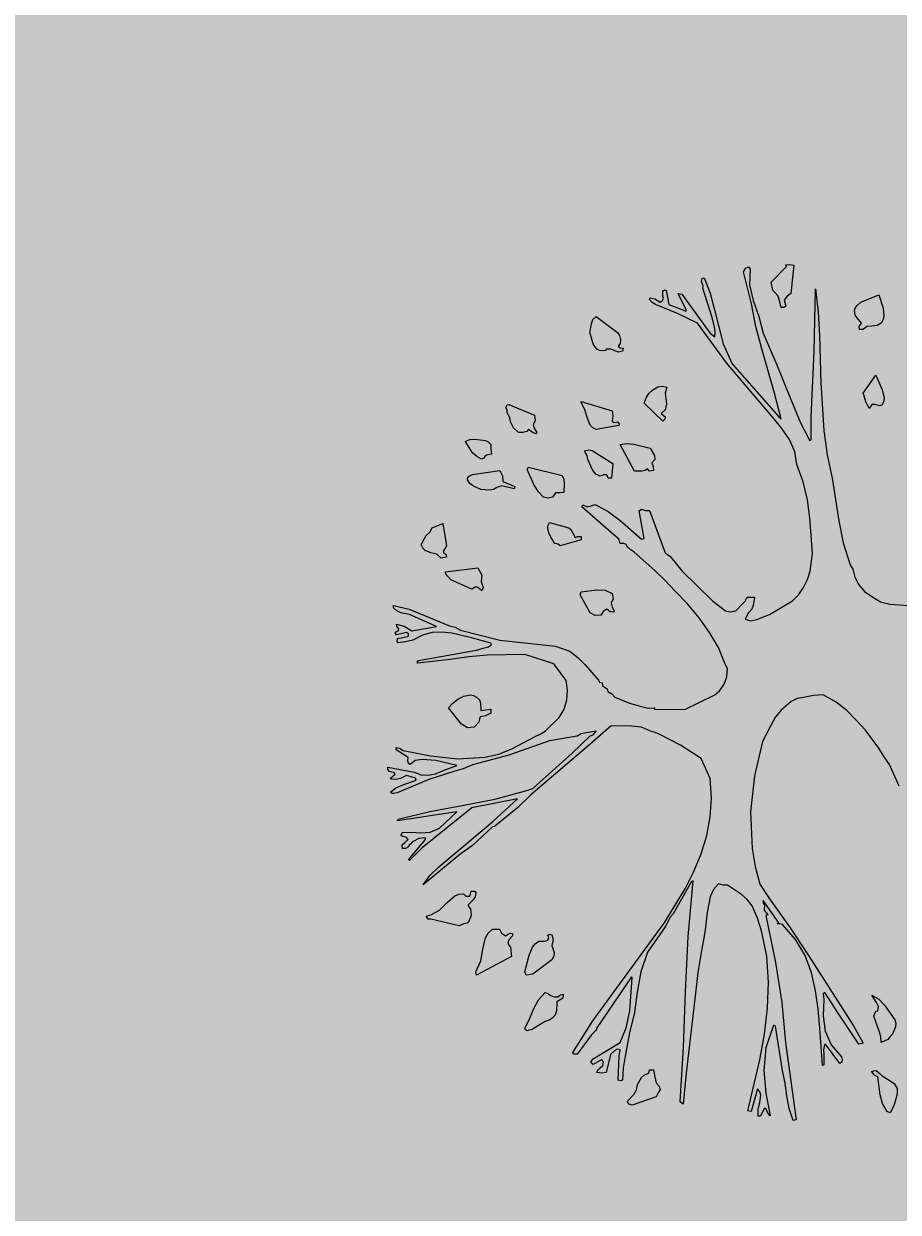
# Model space of a CAD drawing. Units: inches. Extents: x 84 to 1044, y -280 to 906.
# Tile 99 of 105: x 861 to 885, y 445 to 478. Entities that reach past the tile are written whole.
import ezdxf

# ---------------------------------------------------------------- set-up
doc = ezdxf.new("R2010")
doc.units = ezdxf.units.IN
doc.layers.add('A-ANNO-DIMS', color=2, linetype='Continuous', lineweight=18)
doc.layers.add('L-PLNT', color=114, linetype='Continuous', lineweight=15)
doc.layers.add('L-PLNT-PATT', color=9, linetype='Continuous', lineweight=9, true_color=0xafd9aa)
doc.styles.get("Standard").update_dxf_attribs({"font": 'arial.ttf'})
doc.dimstyles.get("Standard").update_dxf_attribs({"dimtxt": 0.18, "dimasz": 0.18, "dimexe": 0.18, "dimexo": 0.0625, "dimgap": 0.09, "dimtad": 0, "dimtih": 1, "dimtoh": 1, "dimdec": 4, "dimzin": 0, "dimdsep": 46, "dimtxsty": 'Standard', "dimcen": 0.09, "dimadec": 0, "dimazin": 0, "dimtfac": 1, "dimtdec": 4, "dimtofl": 0, "dimtmove": 0, "dimatfit": 3, "dimfxl": 1, "dimtolj": 1, "dimtzin": 0, "dimarcsym": 0})

# ---------------------------------------------------------------- blocks, each defined once
blk = doc.blocks.new('A$C37E508DF')
for p, q in [((0.7083, 1.5239), (0.7152, 1.5244)), ((0.7096, 1.5209), (0.7083, 1.5239)), ((0.7152, 1.5244), (0.7225, 1.5231)), ((0.6329, 1.5111), (0.6367, 1.5175)), ((0.6475, 1.4545), (0.6329, 1.5111)), ((0.6367, 1.5175), (0.6423, 1.5201)), ((0.6423, 1.5201), (0.6453, 1.5158)), ((0.6453, 1.5158), (0.644, 1.4879)), ((0.6826, 1.493), (0.7096, 1.5209)), ((0.7225, 1.5231), (0.7174, 1.4729)), ((0.5583, 1.4948), (0.5596, 1.4995)), ((0.5596, 1.4905), (0.5583, 1.4948)), ((0.5596, 1.4995), (0.563, 1.5003)), ((0.5613, 1.4862), (0.5596, 1.4905)), ((0.5608, 1.4823), (0.5613, 1.4862)), ((0.5767, 1.4317), (0.5608, 1.4823)), ((0.563, 1.5003), (0.5737, 1.4733)), ((0.644, 1.4879), (0.6505, 1.46)), ((0.6852, 1.4785), (0.6826, 1.493)), ((0.4657, 1.4622), (0.4669, 1.4652)), ((0.4708, 1.4566), (0.4657, 1.4622)), ((0.4669, 1.4652), (0.4755, 1.463)), ((0.4755, 1.463), (0.4845, 1.4575)), ((0.4884, 1.4596), (0.4905, 1.4635)), ((0.4897, 1.4772), (0.4935, 1.4789)), ((0.4897, 1.4678), (0.4897, 1.4772)), ((0.4905, 1.4635), (0.4897, 1.4678)), ((0.4935, 1.4789), (0.4952, 1.478)), ((0.4952, 1.478), (0.5004, 1.4532)), ((0.5313, 1.4437), (0.5167, 1.4729)), ((0.5167, 1.4729), (0.5231, 1.4716)), ((0.5231, 1.4716), (0.5686, 1.409)), ((0.5737, 1.4733), (0.5814, 1.4437)), ((0.6946, 1.4682), (0.6852, 1.4785)), ((0.6976, 1.4579), (0.6946, 1.4682)), ((0.7109, 1.4682), (0.7053, 1.4609)), ((0.7053, 1.4609), (0.7083, 1.4502)), ((0.7174, 1.4729), (0.7109, 1.4682)), ((0.7589, 1.3691), (0.7615, 1.481)), ((0.7615, 1.481), (0.7658, 1.4395)), ((0.8421, 1.4575), (0.8739, 1.4703)), ((0.8739, 1.4703), (0.882, 1.4463)), ((0.4764, 1.4532), (0.4708, 1.4566)), ((0.5154, 1.4373), (0.4764, 1.4532)), ((0.4845, 1.4575), (0.4884, 1.4596)), ((0.5004, 1.4532), (0.5308, 1.4412)), ((0.5308, 1.4412), (0.5313, 1.4437)), ((0.5814, 1.4437), (0.5969, 1.3833)), ((0.6552, 1.4137), (0.6475, 1.4545)), ((0.6505, 1.46), (0.6603, 1.4317)), ((0.7002, 1.4476), (0.6976, 1.4579)), ((0.7049, 1.448), (0.7002, 1.4476)), ((0.7083, 1.4502), (0.7049, 1.448)), ((0.7658, 1.4395), (0.7684, 1.3979)), ((0.831, 1.4424), (0.8323, 1.4476)), ((0.8318, 1.4343), (0.831, 1.4424)), ((0.8323, 1.4476), (0.8357, 1.451)), ((0.8357, 1.451), (0.8421, 1.4575)), ((0.882, 1.4463), (0.8829, 1.433)), ((0.3598, 1.403), (0.3628, 1.4189)), ((0.3628, 1.4189), (0.3649, 1.4266)), ((0.3649, 1.4266), (0.3709, 1.4317)), ((0.3709, 1.4317), (0.4086, 1.403)), ((0.551, 1.4197), (0.5154, 1.4373)), ((0.6029, 1.3494), (0.551, 1.4197)), ((0.5814, 1.4133), (0.5767, 1.4317)), ((0.6603, 1.4317), (0.668, 1.4021)), ((0.8353, 1.4292), (0.8318, 1.4343)), ((0.8434, 1.4197), (0.8353, 1.4292)), ((0.8391, 1.4141), (0.8434, 1.4197)), ((0.8781, 1.4197), (0.8709, 1.4154)), ((0.8816, 1.4262), (0.8781, 1.4197)), ((0.8829, 1.433), (0.8816, 1.4262)), ((0.3602, 1.4021), (0.3598, 1.403)), ((0.364, 1.3888), (0.3602, 1.4021)), ((0.4086, 1.403), (0.4125, 1.3979)), ((0.4125, 1.3979), (0.4142, 1.391)), ((0.5686, 1.409), (0.5741, 1.4021)), ((0.5741, 1.4021), (0.5823, 1.3953)), ((0.5827, 1.4043), (0.5814, 1.4133)), ((0.5823, 1.3953), (0.5827, 1.4043)), ((0.6655, 1.3743), (0.6552, 1.4137)), ((0.668, 1.4021), (0.6925, 1.3455)), ((0.7684, 1.3979), (0.771, 1.3134)), ((0.8395, 1.4086), (0.8391, 1.4141)), ((0.846, 1.4086), (0.8395, 1.4086)), ((0.8528, 1.4137), (0.846, 1.4086)), ((0.8619, 1.4146), (0.8528, 1.4137)), ((0.8709, 1.4154), (0.8619, 1.4146)), ((0.3657, 1.3828), (0.364, 1.3888)), ((0.3683, 1.3781), (0.3657, 1.3828)), ((0.3718, 1.3738), (0.3683, 1.3781)), ((0.4134, 1.3837), (0.4099, 1.3781)), ((0.4099, 1.3781), (0.4134, 1.376)), ((0.4142, 1.391), (0.4134, 1.3837)), ((0.4134, 1.376), (0.4189, 1.3751)), ((0.5969, 1.3833), (0.6132, 1.3472)), ((0.3765, 1.3713), (0.3718, 1.3738)), ((0.3872, 1.3708), (0.3765, 1.3713)), ((0.3885, 1.3738), (0.3872, 1.3708)), ((0.3971, 1.3734), (0.3885, 1.3738)), ((0.4039, 1.3704), (0.3971, 1.3734)), ((0.4108, 1.3683), (0.4039, 1.3704)), ((0.4176, 1.37), (0.4108, 1.3683)), ((0.4189, 1.3751), (0.4176, 1.37)), ((0.6882, 1.2949), (0.6655, 1.3743)), ((0.7538, 1.2529), (0.7589, 1.3691)), ((0.6595, 1.2829), (0.6029, 1.3494)), ((0.6132, 1.3472), (0.6959, 1.2529)), ((0.6925, 1.3455), (0.7161, 1.2868)), ((0.771, 1.3134), (0.7761, 1.2285)), ((0.846, 1.2949), (0.8687, 1.3271)), ((0.8687, 1.3271), (0.8803, 1.3014)), ((0.4597, 1.2868), (0.4648, 1.2945)), ((0.4648, 1.2945), (0.4717, 1.3009)), ((0.4717, 1.3009), (0.4807, 1.3065)), ((0.4807, 1.3065), (0.4884, 1.3074)), ((0.4884, 1.3074), (0.4965, 1.3057)), ((0.4965, 1.3057), (0.4935, 1.2954)), ((0.4935, 1.2954), (0.4948, 1.2855)), ((0.7002, 1.2495), (0.6882, 1.2949)), ((0.8473, 1.2924), (0.846, 1.2949)), ((0.8507, 1.2795), (0.8473, 1.2924)), ((0.8803, 1.3014), (0.8833, 1.2872)), ((0.2101, 1.2696), (0.2127, 1.2744)), ((0.2127, 1.2744), (0.2152, 1.2752)), ((0.2152, 1.2752), (0.2611, 1.2559)), ((0.3439, 1.2804), (0.3992, 1.2636)), ((0.3439, 1.2787), (0.3439, 1.2804)), ((0.3507, 1.2662), (0.3439, 1.2787)), ((0.4562, 1.2774), (0.4597, 1.2868)), ((0.4897, 1.2452), (0.4562, 1.2774)), ((0.4961, 1.2756), (0.4935, 1.2658)), ((0.4948, 1.2855), (0.4961, 1.2756)), ((0.6865, 1.2508), (0.6595, 1.2829)), ((0.7161, 1.2868), (0.7349, 1.2422)), ((0.8567, 1.2679), (0.8507, 1.2795)), ((0.8619, 1.2752), (0.8567, 1.2679)), ((0.867, 1.2752), (0.8619, 1.2752)), ((0.8713, 1.2739), (0.867, 1.2752)), ((0.8756, 1.2726), (0.8713, 1.2739)), ((0.8799, 1.2744), (0.8756, 1.2726)), ((0.8829, 1.2808), (0.8799, 1.2744)), ((0.8833, 1.2872), (0.8829, 1.2808)), ((0.2127, 1.2654), (0.2101, 1.2696)), ((0.2127, 1.2602), (0.2127, 1.2654)), ((0.2174, 1.2521), (0.2127, 1.2602)), ((0.2182, 1.2443), (0.2174, 1.2521)), ((0.2611, 1.2559), (0.262, 1.2465)), ((0.3546, 1.2516), (0.3507, 1.2662)), ((0.3602, 1.2383), (0.3546, 1.2516)), ((0.3992, 1.2636), (0.4005, 1.2546)), ((0.4005, 1.2546), (0.3992, 1.2452)), ((0.4935, 1.2658), (0.4867, 1.2589)), ((0.4867, 1.2589), (0.4935, 1.2529)), ((0.4931, 1.2491), (0.4897, 1.2452)), ((0.4935, 1.2529), (0.4931, 1.2491)), ((0.7015, 1.2323), (0.6865, 1.2508)), ((0.6959, 1.2529), (0.7002, 1.2495)), ((0.7538, 1.2122), (0.7538, 1.2529)), ((0.2234, 1.2336), (0.2182, 1.2443)), ((0.2328, 1.2251), (0.2234, 1.2336)), ((0.2504, 1.2306), (0.2474, 1.2268)), ((0.2568, 1.2255), (0.2504, 1.2306)), ((0.262, 1.2465), (0.2586, 1.2388)), ((0.2586, 1.2388), (0.2611, 1.2319)), ((0.2611, 1.2319), (0.265, 1.2251)), ((0.3649, 1.2336), (0.3602, 1.2383)), ((0.3709, 1.2306), (0.3649, 1.2336)), ((0.4112, 1.2375), (0.3709, 1.2306)), ((0.3992, 1.2452), (0.4026, 1.2431)), ((0.4026, 1.2431), (0.4086, 1.2443)), ((0.4086, 1.2443), (0.4121, 1.2401)), ((0.4121, 1.2401), (0.4112, 1.2375)), ((0.7148, 1.2126), (0.7015, 1.2323)), ((0.7349, 1.2422), (0.7482, 1.216)), ((0.7761, 1.2285), (0.7821, 1.1856)), ((0.1376, 1.2092), (0.1458, 1.2126)), ((0.1389, 1.2079), (0.1376, 1.2092)), ((0.1505, 1.189), (0.1389, 1.2079)), ((0.1458, 1.2126), (0.1548, 1.2135)), ((0.1548, 1.2135), (0.1741, 1.2109)), ((0.1741, 1.2109), (0.1784, 1.2083)), ((0.1784, 1.2083), (0.1831, 1.204)), ((0.2401, 1.2251), (0.2328, 1.2251)), ((0.2474, 1.2268), (0.2401, 1.2251)), ((0.2633, 1.2229), (0.2568, 1.2255)), ((0.265, 1.2251), (0.2633, 1.2229)), ((0.7246, 1.1908), (0.7148, 1.2126)), ((0.7482, 1.216), (0.7508, 1.2109)), ((0.7508, 1.2109), (0.7538, 1.2122)), ((0.1582, 1.1822), (0.1505, 1.189)), ((0.1788, 1.1852), (0.1758, 1.1847)), ((0.1848, 1.1865), (0.1788, 1.1852)), ((0.1831, 1.204), (0.1831, 1.1959)), ((0.1831, 1.1959), (0.1848, 1.1865)), ((0.3507, 1.1916), (0.352, 1.1933)), ((0.355, 1.1839), (0.3507, 1.1916)), ((0.352, 1.1933), (0.3576, 1.1942)), ((0.3576, 1.1942), (0.364, 1.1929)), ((0.364, 1.1929), (0.4005, 1.1702)), ((0.4134, 1.204), (0.4258, 1.2058)), ((0.4391, 1.156), (0.4134, 1.204)), ((0.4258, 1.2058), (0.4382, 1.2045)), ((0.4382, 1.2045), (0.4669, 1.1972)), ((0.4669, 1.1972), (0.4747, 1.1843)), ((0.7281, 1.168), (0.7246, 1.1908)), ((0.7821, 1.1856), (0.7911, 1.1436)), ((0.1668, 1.1775), (0.1582, 1.1822)), ((0.1711, 1.1792), (0.1668, 1.1775)), ((0.1728, 1.1826), (0.1711, 1.1792)), ((0.1758, 1.1847), (0.1728, 1.1826)), ((0.3563, 1.177), (0.355, 1.1839)), ((0.3645, 1.1586), (0.3563, 1.177)), ((0.4005, 1.1702), (0.3979, 1.1436)), ((0.4751, 1.177), (0.47, 1.1714)), ((0.47, 1.1714), (0.4721, 1.1646)), ((0.4721, 1.1646), (0.473, 1.1573)), ((0.4747, 1.1843), (0.4751, 1.177)), ((0.7396, 1.1371), (0.7281, 1.168)), ((0.1419, 1.1436), (0.1449, 1.1474)), ((0.1419, 1.141), (0.1419, 1.1436)), ((0.1449, 1.1474), (0.1509, 1.1504)), ((0.1509, 1.1504), (0.1994, 1.1573)), ((0.1994, 1.1573), (0.2041, 1.1479)), ((0.2041, 1.1479), (0.2045, 1.138)), ((0.2478, 1.1594), (0.2504, 1.1637)), ((0.2607, 1.1316), (0.2478, 1.1594)), ((0.2504, 1.1637), (0.3104, 1.1487)), ((0.3104, 1.1487), (0.3134, 1.1423)), ((0.37, 1.1509), (0.3645, 1.1586)), ((0.3778, 1.1474), (0.37, 1.1509)), ((0.3842, 1.15), (0.3778, 1.1474)), ((0.3898, 1.15), (0.3842, 1.15)), ((0.3923, 1.1436), (0.3898, 1.15)), ((0.3979, 1.1436), (0.3923, 1.1436)), ((0.4519, 1.1564), (0.4391, 1.156)), ((0.458, 1.1573), (0.4519, 1.1564)), ((0.4622, 1.1607), (0.458, 1.1573)), ((0.4657, 1.156), (0.4622, 1.1607)), ((0.473, 1.1573), (0.4657, 1.156)), ((0.7911, 1.1436), (0.8027, 1.0677)), ((0.1462, 1.1342), (0.1419, 1.141)), ((0.1522, 1.1294), (0.1462, 1.1342)), ((0.1655, 1.1234), (0.1522, 1.1294)), ((0.181, 1.1226), (0.1655, 1.1234)), ((0.1878, 1.1234), (0.181, 1.1226)), ((0.1938, 1.1273), (0.1878, 1.1234)), ((0.2032, 1.1303), (0.1938, 1.1273)), ((0.2247, 1.1251), (0.2032, 1.1303)), ((0.2045, 1.138), (0.226, 1.129)), ((0.226, 1.129), (0.2247, 1.1251)), ((0.268, 1.1196), (0.2607, 1.1316)), ((0.3134, 1.1423), (0.3139, 1.1346)), ((0.3139, 1.1346), (0.3134, 1.1183)), ((0.7469, 1.1054), (0.7396, 1.1371)), ((0.277, 1.1101), (0.268, 1.1196)), ((0.2856, 1.108), (0.277, 1.1101)), ((0.2933, 1.1101), (0.2856, 1.108)), ((0.2959, 1.1144), (0.2933, 1.1101)), ((0.2984, 1.1179), (0.2959, 1.1144)), ((0.3066, 1.1179), (0.2984, 1.1179)), ((0.3134, 1.1183), (0.3066, 1.1179)), ((0.7512, 1.0728), (0.7469, 1.1054)), ((0.3456, 1.093), (0.3469, 1.0964)), ((0.3842, 1.0591), (0.3456, 1.093)), ((0.3469, 1.0964), (0.355, 1.093)), ((0.355, 1.093), (0.3619, 1.0943)), ((0.3619, 1.0943), (0.3692, 1.0968)), ((0.3692, 1.0968), (0.3923, 1.0844)), ((0.3923, 1.0844), (0.4129, 1.069)), ((0.4472, 1.0857), (0.4515, 1.0887)), ((0.4562, 1.0364), (0.4472, 1.0857)), ((0.4515, 1.0887), (0.4584, 1.0865)), ((0.4584, 1.0865), (0.4657, 1.0861)), ((0.4657, 1.0861), (0.4939, 1.0107)), ((0.0789, 1.0552), (0.0978, 1.063)), ((0.0978, 1.063), (0.1042, 1.0231)), ((0.2847, 1.0565), (0.2856, 1.0604)), ((0.2856, 1.0604), (0.2877, 1.0647)), ((0.2877, 1.0647), (0.3224, 1.0552)), ((0.4112, 1.0351), (0.3842, 1.0591)), ((0.4129, 1.069), (0.4515, 1.0351)), ((0.7538, 1.0415), (0.7512, 1.0728)), ((0.8027, 1.0677), (0.8108, 1.0287)), ((0.0596, 1.0257), (0.0682, 1.0415)), ((0.0682, 1.0415), (0.0746, 1.0475)), ((0.0746, 1.0475), (0.0789, 1.0552)), ((0.2851, 1.054), (0.2847, 1.0565)), ((0.2864, 1.0463), (0.2851, 1.054)), ((0.2899, 1.039), (0.2864, 1.0463)), ((0.2972, 1.0274), (0.2899, 1.039)), ((0.3224, 1.0552), (0.3255, 1.0522)), ((0.3255, 1.0522), (0.3293, 1.0458)), ((0.3293, 1.0458), (0.3336, 1.0381)), ((0.3336, 1.0381), (0.3383, 1.0398)), ((0.3383, 1.0398), (0.3439, 1.0402)), ((0.3439, 1.0402), (0.3439, 1.0338)), ((0.7559, 1.0098), (0.7538, 1.0415)), ((0.0626, 1.0188), (0.0596, 1.0257)), ((0.0665, 1.0149), (0.0626, 1.0188)), ((0.1012, 1.018), (0.099, 1.0149)), ((0.1042, 1.0231), (0.1012, 1.018)), ((0.3032, 1.0265), (0.2972, 1.0274)), ((0.3066, 1.0231), (0.3032, 1.0265)), ((0.3439, 1.0338), (0.3066, 1.0231)), ((0.4138, 1.0274), (0.4112, 1.0351)), ((0.4202, 1.0274), (0.4138, 1.0274)), ((0.4241, 1.0257), (0.4202, 1.0274)), ((0.4267, 1.0209), (0.4241, 1.0257)), ((0.4305, 1.0175), (0.4267, 1.0209)), ((0.4378, 1.0124), (0.4305, 1.0175)), ((0.4515, 1.0351), (0.4562, 1.0364)), ((0.8108, 1.0287), (0.8233, 0.9892)), ((0.0763, 1.0111), (0.0665, 1.0149)), ((0.087, 1.0085), (0.0763, 1.0111)), ((0.0948, 1.0016), (0.087, 1.0085)), ((0.1042, 1.0029), (0.0948, 1.0016)), ((0.099, 1.0149), (0.099, 1.0111)), ((0.099, 1.0111), (0.1033, 1.0085)), ((0.1033, 1.0085), (0.1042, 1.0029)), ((0.476, 0.9789), (0.4378, 1.0124)), ((0.4939, 1.0107), (0.5021, 1.0051)), ((0.5021, 1.0051), (0.5094, 0.9969)), ((0.5094, 0.9969), (0.5231, 0.9789)), ((0.7516, 0.9785), (0.7559, 1.0098)), ((0.1025, 0.9751), (0.1029, 0.9772)), ((0.1046, 0.9708), (0.1025, 0.9751)), ((0.1029, 0.9772), (0.1604, 0.9841)), ((0.1604, 0.9841), (0.1672, 0.9708)), ((0.4939, 0.9618), (0.476, 0.9789)), ((0.5231, 0.9789), (0.578, 0.9253)), ((0.7469, 0.9635), (0.7516, 0.9785)), ((0.8233, 0.9892), (0.8275, 0.9815)), ((0.8275, 0.9815), (0.8314, 0.9673)), ((0.1076, 0.9682), (0.1046, 0.9708)), ((0.1119, 0.9626), (0.1076, 0.9682)), ((0.1496, 0.9463), (0.1119, 0.9626)), ((0.1672, 0.9708), (0.1664, 0.9601)), ((0.1664, 0.9601), (0.1698, 0.9493)), ((0.5111, 0.9429), (0.4939, 0.9618)), ((0.7401, 0.9493), (0.7469, 0.9635)), ((0.8314, 0.9673), (0.8383, 0.954)), ((0.8383, 0.954), (0.8486, 0.942)), ((0.1565, 0.9506), (0.1496, 0.9463)), ((0.1604, 0.9493), (0.1565, 0.9506)), ((0.1629, 0.9468), (0.1604, 0.9493)), ((0.1672, 0.9429), (0.1629, 0.9468)), ((0.1698, 0.9493), (0.1672, 0.9429)), ((0.3426, 0.936), (0.3443, 0.9412)), ((0.3602, 0.9039), (0.3426, 0.936)), ((0.3443, 0.9412), (0.3722, 0.9451)), ((0.3722, 0.9451), (0.3868, 0.9446)), ((0.3868, 0.9446), (0.3992, 0.9386)), ((0.3992, 0.9386), (0.4009, 0.9292)), ((0.5334, 0.9202), (0.5111, 0.9429)), ((0.6359, 0.9245), (0.6397, 0.9322)), ((0.6397, 0.9322), (0.653, 0.9322)), ((0.653, 0.9322), (0.6505, 0.9172)), ((0.7203, 0.9253), (0.7315, 0.9365)), ((0.7315, 0.9365), (0.7401, 0.9493)), ((0.8486, 0.942), (0.8619, 0.933)), ((0.8619, 0.933), (0.8769, 0.9236)), ((0.0103, 0.9129), (0.0103, 0.9172)), ((0.0103, 0.9172), (0.0382, 0.9107)), ((0.0159, 0.9073), (0.0103, 0.9129)), ((0.0382, 0.9107), (0.1098, 0.8807)), ((0.3898, 0.9107), (0.3838, 0.9069)), ((0.3958, 0.906), (0.3898, 0.9107)), ((0.4009, 0.9292), (0.3975, 0.9215)), ((0.3975, 0.9215), (0.3996, 0.9142)), ((0.3996, 0.9142), (0.4031, 0.9077)), ((0.554, 0.8953), (0.5334, 0.9202)), ((0.578, 0.9253), (0.6011, 0.9077)), ((0.6196, 0.9077), (0.6303, 0.9189)), ((0.6303, 0.9189), (0.6359, 0.9245)), ((0.6479, 0.9103), (0.6423, 0.9039)), ((0.6505, 0.9172), (0.6479, 0.9103)), ((0.6796, 0.9013), (0.7203, 0.9253)), ((0.8769, 0.9236), (0.8936, 0.9193)), ((0.8936, 0.9193), (0.9279, 0.9172)), ((0.0232, 0.9043), (0.0159, 0.9073)), ((0.0386, 0.9013), (0.0232, 0.9043)), ((0.0866, 0.8794), (0.0386, 0.9013)), ((0.3692, 0.8992), (0.3602, 0.9039)), ((0.379, 0.9), (0.3692, 0.8992)), ((0.3838, 0.9069), (0.379, 0.9)), ((0.4026, 0.9052), (0.3958, 0.906)), ((0.4031, 0.9077), (0.4026, 0.9052)), ((0.5728, 0.8691), (0.554, 0.8953)), ((0.6011, 0.9077), (0.6097, 0.9056)), ((0.6097, 0.9056), (0.6196, 0.9077)), ((0.6384, 0.8974), (0.6359, 0.8927)), ((0.6359, 0.8927), (0.6457, 0.8897)), ((0.6423, 0.9039), (0.6384, 0.8974)), ((0.6457, 0.8897), (0.6569, 0.8919)), ((0.6569, 0.8919), (0.6796, 0.9013)), ((0.0133, 0.8679), (0.015, 0.87)), ((0.0154, 0.8649), (0.0133, 0.8679)), ((0.015, 0.87), (0.0184, 0.8717)), ((0.0159, 0.8803), (0.0154, 0.8837)), ((0.0154, 0.8837), (0.0292, 0.8803)), ((0.0334, 0.8687), (0.0154, 0.8649)), ((0.0176, 0.8777), (0.0159, 0.8803)), ((0.0193, 0.8752), (0.0176, 0.8777)), ((0.0184, 0.8717), (0.0193, 0.8752)), ((0.0292, 0.8803), (0.0424, 0.8717)), ((0.0369, 0.8666), (0.0334, 0.8687)), ((0.0424, 0.8717), (0.0866, 0.8794)), ((0.0789, 0.8687), (0.0617, 0.864)), ((0.0965, 0.8696), (0.0789, 0.8687)), ((0.1141, 0.8679), (0.0965, 0.8696)), ((0.1098, 0.8807), (0.1196, 0.8786)), ((0.1492, 0.8593), (0.1141, 0.8679)), ((0.1196, 0.8786), (0.1295, 0.873)), ((0.1295, 0.873), (0.1994, 0.8554)), ((0.5887, 0.8421), (0.5728, 0.8691)), ((0.0163, 0.8529), (0.0171, 0.8584)), ((0.0184, 0.8503), (0.0163, 0.8529)), ((0.0171, 0.8584), (0.0266, 0.8602)), ((0.0317, 0.8524), (0.0184, 0.8503)), ((0.0266, 0.8602), (0.0369, 0.8623)), ((0.0442, 0.8554), (0.0317, 0.8524)), ((0.0369, 0.8623), (0.0369, 0.8666)), ((0.0617, 0.864), (0.0442, 0.8554)), ((0.1835, 0.8499), (0.1492, 0.8593)), ((0.1792, 0.8434), (0.1848, 0.8477)), ((0.1848, 0.8477), (0.1835, 0.8499)), ((0.1994, 0.8554), (0.2984, 0.8447)), ((0.0545, 0.8194), (0.1578, 0.8378)), ((0.1441, 0.8258), (0.1111, 0.8207)), ((0.1771, 0.8288), (0.1441, 0.8258)), ((0.1578, 0.8378), (0.1698, 0.8413)), ((0.1698, 0.8413), (0.1792, 0.8434)), ((0.2436, 0.8301), (0.1771, 0.8288)), ((0.2954, 0.813), (0.2436, 0.8301)), ((0.2984, 0.8447), (0.3242, 0.8357)), ((0.3242, 0.8357), (0.3387, 0.8241)), ((0.6007, 0.8125), (0.5887, 0.8421)), ((0.0519, 0.8164), (0.0545, 0.8194)), ((0.0532, 0.8143), (0.0519, 0.8164)), ((0.1111, 0.8207), (0.0532, 0.8143)), ((0.3173, 0.7834), (0.2954, 0.813)), ((0.3387, 0.8241), (0.3512, 0.8117)), ((0.3512, 0.8117), (0.3748, 0.7842)), ((0.6046, 0.8048), (0.6007, 0.8125)), ((0.6037, 0.7903), (0.6046, 0.8048)), ((0.3199, 0.7662), (0.3173, 0.7834)), ((0.3748, 0.7842), (0.3765, 0.7804)), ((0.599, 0.777), (0.6037, 0.7903)), ((0.3186, 0.7491), (0.3199, 0.7662)), ((0.3765, 0.7804), (0.3816, 0.7791)), ((0.3816, 0.7791), (0.382, 0.7744)), ((0.382, 0.7744), (0.3859, 0.7714)), ((0.3859, 0.7714), (0.3902, 0.7684)), ((0.3902, 0.7684), (0.3919, 0.7641)), ((0.3919, 0.7641), (0.3988, 0.7598)), ((0.5823, 0.7577), (0.5913, 0.7658)), ((0.5913, 0.7658), (0.599, 0.777)), ((0.1081, 0.7349), (0.1153, 0.7427)), ((0.1153, 0.7427), (0.1244, 0.7504)), ((0.1244, 0.7504), (0.1351, 0.7559)), ((0.1351, 0.7559), (0.1471, 0.7577)), ((0.1471, 0.7577), (0.1527, 0.7568)), ((0.1527, 0.7568), (0.1578, 0.7538)), ((0.1578, 0.7538), (0.1629, 0.7491)), ((0.1629, 0.7491), (0.1651, 0.7431)), ((0.1651, 0.7431), (0.1655, 0.7298)), ((0.3139, 0.7324), (0.3186, 0.7491)), ((0.3988, 0.7598), (0.4043, 0.7538)), ((0.4043, 0.7538), (0.4301, 0.7431)), ((0.4301, 0.7431), (0.4515, 0.7371)), ((0.5287, 0.7319), (0.5823, 0.7577)), ((0.7182, 0.7461), (0.7002, 0.7307)), ((0.7285, 0.7512), (0.7182, 0.7461)), ((0.7401, 0.7534), (0.7285, 0.7512)), ((0.7577, 0.7568), (0.7401, 0.7534)), ((0.7752, 0.7577), (0.7577, 0.7568)), ((0.798, 0.7452), (0.7752, 0.7577)), ((0.8173, 0.7298), (0.798, 0.7452)), ((0.1312, 0.7058), (0.1081, 0.7349)), ((0.1741, 0.7208), (0.1646, 0.7186)), ((0.1655, 0.7298), (0.1831, 0.7324)), ((0.1831, 0.7255), (0.1741, 0.7208)), ((0.1831, 0.7324), (0.1831, 0.7255)), ((0.3049, 0.7178), (0.3139, 0.7324)), ((0.4515, 0.7371), (0.4635, 0.7341)), ((0.4635, 0.7341), (0.4755, 0.7349)), ((0.4755, 0.7349), (0.4742, 0.7324)), ((0.4742, 0.7324), (0.5287, 0.7319)), ((0.7002, 0.7307), (0.6903, 0.7186)), ((0.8344, 0.7122), (0.8173, 0.7298)), ((0.1415, 0.6994), (0.1312, 0.7058)), ((0.1539, 0.7002), (0.1415, 0.6994)), ((0.1621, 0.7092), (0.1539, 0.7002)), ((0.1629, 0.7152), (0.1621, 0.7092)), ((0.1646, 0.7186), (0.1629, 0.7152)), ((0.28, 0.6933), (0.3049, 0.7178)), ((0.3975, 0.7028), (0.3598, 0.6693)), ((0.4339, 0.7019), (0.3975, 0.7028)), ((0.4515, 0.7002), (0.4339, 0.7019)), ((0.4674, 0.6933), (0.4515, 0.7002)), ((0.6818, 0.7032), (0.6667, 0.6749)), ((0.6903, 0.7186), (0.6818, 0.7032)), ((0.8503, 0.6951), (0.8344, 0.7122)), ((0.2221, 0.6625), (0.262, 0.6839)), ((0.262, 0.6839), (0.271, 0.6882)), ((0.271, 0.6882), (0.28, 0.6933)), ((0.337, 0.6843), (0.2877, 0.6762)), ((0.328, 0.6543), (0.3598, 0.6843)), ((0.3443, 0.6886), (0.337, 0.6843)), ((0.3533, 0.6903), (0.3443, 0.6886)), ((0.3709, 0.6933), (0.3533, 0.6903)), ((0.3598, 0.6843), (0.3662, 0.6873)), ((0.3662, 0.6873), (0.3709, 0.6933)), ((0.476, 0.6912), (0.4674, 0.6933)), ((0.4832, 0.6878), (0.476, 0.6912)), ((0.521, 0.6685), (0.4832, 0.6878)), ((0.8739, 0.6629), (0.8503, 0.6951)), ((0.0146, 0.6599), (0.0146, 0.6642)), ((0.0146, 0.6642), (0.0206, 0.6633)), ((0.036, 0.6466), (0.0146, 0.6599)), ((0.0206, 0.6633), (0.0274, 0.6586)), ((0.0274, 0.6586), (0.0759, 0.6492)), ((0.1977, 0.6526), (0.2221, 0.6625)), ((0.2877, 0.6762), (0.2152, 0.6505)), ((0.3598, 0.6693), (0.2543, 0.5797)), ((0.5578, 0.6449), (0.521, 0.6685)), ((0.6667, 0.6749), (0.6526, 0.614)), ((0.8824, 0.6492), (0.8739, 0.6629)), ((0.0356, 0.6406), (0.036, 0.6466)), ((0.0369, 0.6355), (0.0356, 0.6406)), ((0.0399, 0.6342), (0.0369, 0.6355)), ((0.0489, 0.641), (0.0399, 0.6342)), ((0.0609, 0.6428), (0.0489, 0.641)), ((0.0853, 0.641), (0.0609, 0.6428)), ((0.0759, 0.6492), (0.1244, 0.644)), ((0.1226, 0.632), (0.0853, 0.641)), ((0.1244, 0.644), (0.1728, 0.647)), ((0.2152, 0.6505), (0.1509, 0.6333)), ((0.1728, 0.647), (0.1977, 0.6526)), ((0.2581, 0.5913), (0.328, 0.6543)), ((0.5737, 0.6089), (0.5578, 0.6449)), ((0.8932, 0.6342), (0.8824, 0.6492)), ((0, 0.629), (0.0467, 0.62)), ((0, 0.6252), (0, 0.629)), ((0.003, 0.6213), (0, 0.6252)), ((0.0069, 0.6204), (0.003, 0.6213)), ((0.0107, 0.6196), (0.0069, 0.6204)), ((0.0086, 0.6132), (0.0133, 0.617)), ((0.0133, 0.617), (0.0107, 0.6196)), ((0.0334, 0.6145), (0.0223, 0.6089)), ((0.0416, 0.6119), (0.0334, 0.6145)), ((0.0467, 0.62), (0.0592, 0.6153)), ((0.0592, 0.6153), (0.072, 0.6149)), ((0.072, 0.6149), (0.0849, 0.6175)), ((0.1175, 0.6213), (0.0746, 0.6076)), ((0.0849, 0.6175), (0.0973, 0.6226)), ((0.0973, 0.6226), (0.1226, 0.632)), ((0.1342, 0.6265), (0.1175, 0.6213)), ((0.1509, 0.6333), (0.1342, 0.6265)), ((0.6526, 0.614), (0.6457, 0.5497)), ((0.9103, 0.5956), (0.8932, 0.6342)), ((0.0047, 0.6093), (0.0086, 0.6132)), ((0.0056, 0.6076), (0.0047, 0.6093)), ((0.0141, 0.6072), (0.0056, 0.6076)), ((0.0223, 0.6089), (0.0141, 0.6072)), ((0.0141, 0.5921), (0.0257, 0.5969)), ((0.0746, 0.6076), (0.0163, 0.5836)), ((0.0257, 0.5969), (0.0506, 0.6063)), ((0.0493, 0.6093), (0.0416, 0.6119)), ((0.0506, 0.6063), (0.0493, 0.6093)), ((0.5763, 0.5741), (0.5737, 0.6089)), ((0.0047, 0.5849), (0.0141, 0.5921)), ((0.0069, 0.5823), (0.0047, 0.5849)), ((0.0099, 0.5823), (0.0069, 0.5823)), ((0.0163, 0.5836), (0.0099, 0.5823)), ((0.1325, 0.5608), (0.1904, 0.5724)), ((0.2311, 0.5729), (0.1496, 0.557)), ((0.1869, 0.5325), (0.2311, 0.5729)), ((0.1904, 0.5724), (0.2474, 0.5879)), ((0.2543, 0.5797), (0.2311, 0.557)), ((0.2474, 0.5879), (0.253, 0.5892)), ((0.253, 0.5892), (0.2581, 0.5913)), ((0.5737, 0.5407), (0.5763, 0.5741)), ((0.1496, 0.557), (0.0613, 0.4858)), ((0.0746, 0.5501), (0.1325, 0.5608)), ((0.2311, 0.557), (0.1899, 0.5235)), ((0.1226, 0.5497), (0.0171, 0.5338)), ((0.0171, 0.5338), (0.0184, 0.5368)), ((0.0184, 0.5368), (0.0746, 0.5501)), ((0.0917, 0.5205), (0.1226, 0.5497)), ((0.1269, 0.482), (0.1869, 0.5325)), ((0.5677, 0.5077), (0.5737, 0.5407)), ((0.6457, 0.5497), (0.6483, 0.4845)), ((0.024, 0.5072), (0.0253, 0.5128)), ((0.0253, 0.5128), (0.042, 0.5133)), ((0.042, 0.5133), (0.0587, 0.5124)), ((0.0587, 0.5124), (0.0755, 0.5133)), ((0.0755, 0.5133), (0.0917, 0.5205)), ((0.1861, 0.5231), (0.1509, 0.4897)), ((0.1899, 0.5235), (0.1861, 0.5231)), ((0.0262, 0.5055), (0.024, 0.5072)), ((0.0253, 0.491), (0.03, 0.4948)), ((0.0262, 0.4841), (0.0253, 0.491)), ((0.0326, 0.5047), (0.0262, 0.5055)), ((0.03, 0.4948), (0.036, 0.5004)), ((0.0369, 0.4871), (0.0317, 0.4841)), ((0.036, 0.5004), (0.0326, 0.5047)), ((0.0369, 0.4639), (0.0669, 0.5004)), ((0.0382, 0.4905), (0.0369, 0.4871)), ((0.0403, 0.4922), (0.0382, 0.4905)), ((0.0437, 0.4961), (0.0403, 0.4922)), ((0.0549, 0.5021), (0.0437, 0.4961)), ((0.0669, 0.5034), (0.0549, 0.5021)), ((0.0669, 0.5004), (0.0669, 0.5034)), ((0.1509, 0.4897), (0.1282, 0.4734)), ((0.5578, 0.4751), (0.5677, 0.5077)), ((0.0317, 0.4841), (0.0262, 0.4841)), ((0.0613, 0.4858), (0.0386, 0.4627)), ((0.1282, 0.4734), (0.0626, 0.4198)), ((0.0905, 0.4515), (0.1269, 0.482)), ((0.545, 0.4434), (0.5578, 0.4751)), ((0.6483, 0.4845), (0.6539, 0.4524)), ((0.0386, 0.4627), (0.0369, 0.4639)), ((0.0746, 0.4361), (0.0905, 0.4515)), ((0.6539, 0.4524), (0.6625, 0.4211)), ((0.0626, 0.4198), (0.0746, 0.4361)), ((0.5403, 0.4254), (0.5081, 0.3679)), ((0.5295, 0.4125), (0.545, 0.4434)), ((0.5347, 0.3276), (0.5433, 0.4266)), ((0.5433, 0.4266), (0.5403, 0.4254)), ((0.1192, 0.4001), (0.1265, 0.4031)), ((0.1265, 0.4031), (0.1346, 0.4039)), ((0.1346, 0.4039), (0.1389, 0.3992)), ((0.1458, 0.3996), (0.1471, 0.4035)), ((0.1471, 0.4035), (0.1484, 0.4082)), ((0.1484, 0.4082), (0.1548, 0.4082)), ((0.1548, 0.4082), (0.1565, 0.4052)), ((0.1565, 0.4052), (0.1556, 0.3983)), ((0.4922, 0.3516), (0.5295, 0.4125)), ((0.5797, 0.4112), (0.5741, 0.3983)), ((0.5887, 0.4215), (0.5797, 0.4112)), ((0.5969, 0.4189), (0.5887, 0.4215)), ((0.6046, 0.4189), (0.5969, 0.4189)), ((0.6295, 0.4022), (0.6046, 0.4189)), ((0.6397, 0.3936), (0.6295, 0.4022)), ((0.6625, 0.4211), (0.6796, 0.3945)), ((0.0917, 0.3748), (0.1055, 0.388)), ((0.1055, 0.388), (0.1192, 0.4001)), ((0.1389, 0.3992), (0.1458, 0.3996)), ((0.1518, 0.3932), (0.1432, 0.3842)), ((0.1432, 0.3842), (0.1436, 0.3808)), ((0.1556, 0.3983), (0.1518, 0.3932)), ((0.5741, 0.3983), (0.5686, 0.3705)), ((0.6487, 0.3825), (0.6397, 0.3936)), ((0.6582, 0.3602), (0.6487, 0.3825)), ((0.6959, 0.352), (0.668, 0.3919)), ((0.668, 0.3919), (0.668, 0.3872)), ((0.668, 0.3872), (0.6706, 0.3842)), ((0.6706, 0.3842), (0.6702, 0.3748)), ((0.6796, 0.3945), (0.7148, 0.3447)), ((0.069, 0.364), (0.0763, 0.3662)), ((0.069, 0.3627), (0.069, 0.364)), ((0.0716, 0.3585), (0.069, 0.3627)), ((0.0763, 0.3662), (0.0917, 0.3748)), ((0.1484, 0.3649), (0.1432, 0.352)), ((0.1436, 0.3808), (0.1471, 0.3769)), ((0.1471, 0.3769), (0.1484, 0.3649)), ((0.5025, 0.3619), (0.4982, 0.3537)), ((0.5081, 0.3679), (0.5025, 0.3619)), ((0.5686, 0.3705), (0.5643, 0.3349)), ((0.665, 0.3379), (0.6582, 0.3602)), ((0.6702, 0.3748), (0.6762, 0.3662)), ((0.6762, 0.3662), (0.6732, 0.3653)), ((0.6732, 0.3653), (0.6903, 0.2813)), ((0.0763, 0.3585), (0.0716, 0.3585)), ((0.1269, 0.3464), (0.0763, 0.3585)), ((0.1355, 0.3499), (0.1269, 0.3464)), ((0.1432, 0.352), (0.1355, 0.3499)), ((0.1788, 0.3336), (0.1861, 0.3409)), ((0.1861, 0.3409), (0.199, 0.3409)), ((0.199, 0.3409), (0.2024, 0.3336)), ((0.4065, 0.2345), (0.4922, 0.3516)), ((0.4939, 0.3447), (0.4884, 0.337)), ((0.4982, 0.3537), (0.4939, 0.3447)), ((0.6933, 0.3503), (0.6959, 0.352)), ((0.6985, 0.3503), (0.6933, 0.3503)), ((0.7023, 0.349), (0.6985, 0.3503)), ((0.7259, 0.3224), (0.7023, 0.349)), ((0.7148, 0.3447), (0.7487, 0.2937)), ((0.1689, 0.3053), (0.1737, 0.325)), ((0.1737, 0.325), (0.1788, 0.3336)), ((0.2024, 0.3336), (0.2097, 0.3289)), ((0.2097, 0.3289), (0.2148, 0.3323)), ((0.2161, 0.3224), (0.214, 0.3186)), ((0.214, 0.3186), (0.214, 0.3139)), ((0.2148, 0.3323), (0.2182, 0.3336)), ((0.2221, 0.3289), (0.2161, 0.3224)), ((0.2182, 0.3336), (0.2221, 0.3327)), ((0.2221, 0.3327), (0.2221, 0.3289)), ((0.2624, 0.3147), (0.2689, 0.3194)), ((0.2689, 0.3194), (0.2796, 0.3194)), ((0.2796, 0.3194), (0.2847, 0.3211)), ((0.2847, 0.3211), (0.2864, 0.325)), ((0.2851, 0.3302), (0.2877, 0.3319)), ((0.2864, 0.325), (0.2851, 0.3302)), ((0.2877, 0.3319), (0.292, 0.3306)), ((0.292, 0.3306), (0.2941, 0.322)), ((0.2941, 0.322), (0.292, 0.3117)), ((0.4884, 0.337), (0.4622, 0.2997)), ((0.53, 0.229), (0.5347, 0.3276)), ((0.5643, 0.3349), (0.5578, 0.2993)), ((0.6745, 0.2924), (0.665, 0.3379)), ((0.7427, 0.2937), (0.7259, 0.3224)), ((0.1655, 0.2843), (0.1689, 0.3053)), ((0.214, 0.3139), (0.2182, 0.3087)), ((0.2182, 0.3087), (0.2204, 0.292)), ((0.2517, 0.2946), (0.2577, 0.3087)), ((0.2577, 0.3087), (0.2624, 0.3147)), ((0.292, 0.3117), (0.2959, 0.2993)), ((0.2959, 0.2993), (0.2954, 0.2928)), ((0.4622, 0.2997), (0.4502, 0.2645)), ((0.5578, 0.2993), (0.5518, 0.2633)), ((0.1565, 0.265), (0.1655, 0.2843)), ((0.2204, 0.292), (0.1578, 0.259)), ((0.2436, 0.265), (0.2517, 0.2946)), ((0.292, 0.286), (0.2581, 0.2607)), ((0.2954, 0.2928), (0.292, 0.286)), ((0.6775, 0.2465), (0.6745, 0.2924)), ((0.6903, 0.2813), (0.7015, 0.2101)), ((0.7542, 0.2628), (0.7427, 0.2937)), ((0.7487, 0.2937), (0.8151, 0.1899)), ((0.1578, 0.259), (0.1565, 0.265)), ((0.2461, 0.259), (0.2436, 0.265)), ((0.2581, 0.2607), (0.2461, 0.259)), ((0.4335, 0.2556), (0.3709, 0.1634)), ((0.4305, 0.1951), (0.4352, 0.2543)), ((0.4352, 0.2543), (0.4335, 0.2556)), ((0.4502, 0.2645), (0.4438, 0.2285)), ((0.5518, 0.2633), (0.5475, 0.2268)), ((0.7615, 0.2311), (0.7542, 0.2628)), ((0.3649, 0.1775), (0.4065, 0.2345)), ((0.6758, 0.2002), (0.6775, 0.2465)), ((0.2594, 0.1981), (0.268, 0.2148)), ((0.268, 0.2148), (0.28, 0.2277)), ((0.28, 0.2277), (0.2851, 0.226)), ((0.2851, 0.226), (0.2903, 0.2225)), ((0.2903, 0.2225), (0.2963, 0.22)), ((0.2963, 0.22), (0.3027, 0.2204)), ((0.3096, 0.2165), (0.301, 0.211)), ((0.3027, 0.2204), (0.3061, 0.2234)), ((0.3061, 0.2234), (0.3122, 0.2247)), ((0.3122, 0.22), (0.3096, 0.2165)), ((0.3122, 0.2247), (0.3122, 0.22)), ((0.4438, 0.2285), (0.4391, 0.1921)), ((0.5261, 0.1308), (0.53, 0.229)), ((0.5475, 0.2268), (0.5313, 0.084)), ((0.7662, 0.1981), (0.7615, 0.2311)), ((0.7778, 0.2277), (0.7752, 0.2255)), ((0.7752, 0.2255), (0.7761, 0.2152)), ((0.7761, 0.2152), (0.7752, 0.1861)), ((0.8018, 0.1912), (0.7778, 0.2277)), ((0.8619, 0.2234), (0.8739, 0.2161)), ((0.87, 0.2101), (0.8619, 0.2234)), ((0.8739, 0.2161), (0.8841, 0.2054)), ((0.2521, 0.1805), (0.2594, 0.1981)), ((0.3002, 0.1951), (0.298, 0.1874)), ((0.301, 0.211), (0.3002, 0.1951)), ((0.4241, 0.1651), (0.4305, 0.1951)), ((0.4391, 0.1921), (0.4301, 0.1561)), ((0.6706, 0.1539), (0.6758, 0.2002)), ((0.7015, 0.2101), (0.7079, 0.1389)), ((0.7688, 0.1646), (0.7662, 0.1981)), ((0.8383, 0.1359), (0.8018, 0.1912)), ((0.8649, 0.1857), (0.8687, 0.1947)), ((0.8687, 0.1947), (0.8726, 0.1955)), ((0.8734, 0.2032), (0.87, 0.2101)), ((0.8726, 0.1955), (0.8734, 0.2032)), ((0.8841, 0.2054), (0.9026, 0.1792)), ((0.2436, 0.1642), (0.2521, 0.1805)), ((0.28, 0.1762), (0.2684, 0.1689)), ((0.2873, 0.1788), (0.28, 0.1762)), ((0.292, 0.1818), (0.2873, 0.1788)), ((0.298, 0.1874), (0.292, 0.1818)), ((0.3293, 0.1213), (0.3649, 0.1775)), ((0.6865, 0.1698), (0.6732, 0.1295)), ((0.6903, 0.1681), (0.6865, 0.1698)), ((0.7752, 0.1861), (0.7787, 0.1591)), ((0.8151, 0.1899), (0.8288, 0.1685)), ((0.8743, 0.1608), (0.8649, 0.1857)), ((0.9026, 0.1792), (0.9043, 0.1732)), ((0.9043, 0.1732), (0.9035, 0.1668)), ((0.2448, 0.1616), (0.2436, 0.1642)), ((0.2478, 0.1599), (0.2448, 0.1616)), ((0.2508, 0.1608), (0.2478, 0.1599)), ((0.2556, 0.1616), (0.2508, 0.1608)), ((0.2684, 0.1689), (0.2556, 0.1616)), ((0.3628, 0.1526), (0.337, 0.1183)), ((0.3692, 0.1591), (0.3628, 0.1526)), ((0.3718, 0.1616), (0.3692, 0.1591)), ((0.3709, 0.1634), (0.3718, 0.1616)), ((0.4138, 0.1389), (0.4241, 0.1651)), ((0.4301, 0.1561), (0.4224, 0.1145)), ((0.662, 0.108), (0.6706, 0.1539)), ((0.7023, 0.0892), (0.6903, 0.1681)), ((0.774, 0.0982), (0.7688, 0.1646)), ((0.7787, 0.1591), (0.789, 0.1346)), ((0.8288, 0.1685), (0.846, 0.1376)), ((0.8777, 0.1496), (0.8743, 0.1608)), ((0.8781, 0.1389), (0.8777, 0.1496)), ((0.894, 0.1496), (0.8902, 0.1441)), ((0.8983, 0.1535), (0.894, 0.1496)), ((0.9035, 0.1668), (0.8983, 0.1535)), ((0.3653, 0.1098), (0.4138, 0.1389)), ((0.5205, 0.033), (0.5261, 0.1308)), ((0.6732, 0.1295), (0.6693, 0.0892)), ((0.7079, 0.1389), (0.7268, 0.0013)), ((0.7774, 0.1346), (0.7757, 0.1261)), ((0.7791, 0.1359), (0.7774, 0.1346)), ((0.8044, 0.1012), (0.7791, 0.1359)), ((0.789, 0.1346), (0.8074, 0.1132)), ((0.846, 0.1376), (0.8383, 0.1359)), ((0.8846, 0.1419), (0.8781, 0.1389)), ((0.8902, 0.1441), (0.8846, 0.1419)), ((0.3306, 0.1183), (0.3293, 0.1213)), ((0.337, 0.1183), (0.3306, 0.1183)), ((0.3615, 0.1042), (0.3653, 0.1098)), ((0.3812, 0.1089), (0.3653, 0.0999)), ((0.3842, 0.1037), (0.3812, 0.1089)), ((0.3962, 0.1175), (0.3885, 0.0853)), ((0.4039, 0.1248), (0.3962, 0.1175)), ((0.4082, 0.1269), (0.4039, 0.1248)), ((0.4134, 0.1256), (0.4082, 0.1269)), ((0.4099, 0.0716), (0.4121, 0.1145)), ((0.4121, 0.1145), (0.4134, 0.1256)), ((0.4224, 0.1145), (0.4189, 0.093)), ((0.641, 0.0172), (0.662, 0.108)), ((0.7757, 0.1261), (0.7761, 0.117)), ((0.7761, 0.117), (0.7761, 0.099)), ((0.8074, 0.1132), (0.8087, 0.1089)), ((0.8087, 0.1089), (0.8083, 0.1037)), ((0.3653, 0.0999), (0.3615, 0.1042)), ((0.3722, 0.0853), (0.3739, 0.09)), ((0.3808, 0.0845), (0.3722, 0.0853)), ((0.3739, 0.09), (0.3782, 0.0935)), ((0.3782, 0.0935), (0.3825, 0.0978)), ((0.3885, 0.0853), (0.3808, 0.0845)), ((0.3825, 0.0978), (0.3842, 0.1037)), ((0.4189, 0.093), (0.4176, 0.072)), ((0.4648, 0.084), (0.4657, 0.0905)), ((0.4657, 0.0905), (0.473, 0.0905)), ((0.473, 0.0905), (0.476, 0.0746)), ((0.6693, 0.0892), (0.6728, 0.0484)), ((0.7075, 0.0665), (0.7023, 0.0892)), ((0.7761, 0.099), (0.774, 0.0982)), ((0.8083, 0.1037), (0.8044, 0.1012)), ((0.8619, 0.0875), (0.8649, 0.0887)), ((0.8619, 0.0866), (0.8619, 0.0875)), ((0.8666, 0.0806), (0.8619, 0.0866)), ((0.8649, 0.0887), (0.8691, 0.0892)), ((0.8691, 0.0892), (0.8769, 0.0827)), ((0.4142, 0.0707), (0.4099, 0.0716)), ((0.4176, 0.072), (0.4142, 0.0707)), ((0.4425, 0.0544), (0.4442, 0.0639)), ((0.4442, 0.0639), (0.4515, 0.0763)), ((0.4515, 0.0763), (0.4571, 0.0815)), ((0.4571, 0.0815), (0.4648, 0.084)), ((0.476, 0.0746), (0.4777, 0.0673)), ((0.4777, 0.0673), (0.4832, 0.0613)), ((0.5313, 0.084), (0.5257, 0.0291)), ((0.7105, 0.0437), (0.7075, 0.0665)), ((0.8726, 0.0776), (0.8666, 0.0806)), ((0.8764, 0.0459), (0.8726, 0.0776)), ((0.8769, 0.0827), (0.8799, 0.0797)), ((0.8799, 0.0797), (0.8893, 0.0733)), ((0.8893, 0.0733), (0.9013, 0.066)), ((0.9013, 0.066), (0.9069, 0.057)), ((0.4258, 0.0339), (0.4378, 0.0463)), ((0.4777, 0.0424), (0.4348, 0.0274)), ((0.4378, 0.0463), (0.4425, 0.0544)), ((0.4811, 0.0493), (0.4777, 0.0424)), ((0.4845, 0.0553), (0.4811, 0.0493)), ((0.4832, 0.0613), (0.4845, 0.0553)), ((0.6582, 0.0562), (0.6466, 0.0159)), ((0.6625, 0.051), (0.6582, 0.0562)), ((0.6642, 0.045), (0.6625, 0.051)), ((0.6625, 0.0321), (0.6642, 0.045)), ((0.6728, 0.0484), (0.6809, 0.0082)), ((0.7144, 0.0214), (0.7105, 0.0437)), ((0.8807, 0.0304), (0.8764, 0.0459)), ((0.9069, 0.0471), (0.9009, 0.0261)), ((0.9069, 0.057), (0.9069, 0.0471)), ((0.4296, 0.0291), (0.4258, 0.0339)), ((0.4348, 0.0274), (0.4296, 0.0291)), ((0.5257, 0.0291), (0.5205, 0.033)), ((0.659, 0.0193), (0.6625, 0.0321)), ((0.6702, 0.0214), (0.6637, 0.0077)), ((0.6732, 0.0214), (0.6702, 0.0214)), ((0.6766, 0.0133), (0.6732, 0.0214)), ((0.7216, 0), (0.7144, 0.0214)), ((0.8889, 0.0159), (0.8807, 0.0304)), ((0.9009, 0.0261), (0.894, 0.0137)), ((0.6466, 0.0159), (0.641, 0.0172)), ((0.6595, 0.0077), (0.659, 0.0193)), ((0.6637, 0.0077), (0.6595, 0.0077)), ((0.6809, 0.0082), (0.6766, 0.0133)), ((0.7268, 0.0013), (0.7216, 0)), ((0.894, 0.0137), (0.8889, 0.0159))]:
    blk.add_line(p, q)
blk = doc.blocks.new('*D62')
at = {"layer": 'A-ANNO-DIMS', "color": 0, "lineweight": -2, "transparency": 16777216}
for p, q in [((203.179, 709.183), (203.179, 905.9)), ((203.359, 905.72), (549.232, 905.72)), ((895.894, 905.72), (550.021, 905.72)), ((896.074, 400.183), (896.074, 905.9))]:
    blk.add_line(p, q, dxfattribs=at)
at = {"layer": 'A-ANNO-DIMS', "color": 0, "transparency": 16777216}
for points in [[(203.359, 905.75), (203.359, 905.69), (203.179, 905.72)], [(895.894, 905.75), (895.894, 905.69), (896.074, 905.72)]]:
    blk.add_solid(points, dxfattribs=at)
at = {"layer": 'Defpoints', "color": 0, "transparency": 16777216}
for p in [(896.074, 905.72), (203.179, 709.12), (896.074, 400.12)]:
    blk.add_point(p, dxfattribs=at)
at = {"layer": 'A-ANNO-DIMS', "color": 0, "transparency": 16777216, "insert": (549.627, 905.72), "char_height": 0.18, "attachment_point": 5}
blk.add_mtext('\\A1;692.9', dxfattribs=at)
blk = doc.blocks.new('*D63')
at = {"layer": 'A-ANNO-DIMS', "color": 0, "lineweight": -2, "transparency": 16777216}
for p, q in [((833.136, 709.12), (1043.768, 709.12)), ((1043.588, 708.94), (1043.588, 400.302)), ((1043.588, 91.3), (1043.588, 399.938)), ((896.136, 91.12), (1043.768, 91.12))]:
    blk.add_line(p, q, dxfattribs=at)
at = {"layer": 'A-ANNO-DIMS', "color": 0, "transparency": 16777216}
for points in [[(1043.558, 708.94), (1043.618, 708.94), (1043.588, 709.12)], [(1043.558, 91.3), (1043.618, 91.3), (1043.588, 91.12)]]:
    blk.add_solid(points, dxfattribs=at)
at = {"layer": 'Defpoints', "color": 0, "transparency": 16777216}
for p in [(833.074, 709.12), (1043.588, 709.12), (896.074, 91.12)]:
    blk.add_point(p, dxfattribs=at)
at = {"layer": 'A-ANNO-DIMS', "color": 0, "transparency": 16777216, "insert": (1043.588, 400.12), "char_height": 0.18, "attachment_point": 5}
blk.add_mtext('\\A1;618', dxfattribs=at)

msp = doc.modelspace()

# ---------------------------------------------------------------- hatches: boundary and pattern name
at = {"layer": 'L-PLNT-PATT', "transparency": 33554597}
h = msp.add_hatch(color=256, dxfattribs=at)
h.dxf.hatch_style = 1
h.paths.add_polyline_path([(896.074, 511.12), (704.074, 511.12), (704.074, 491.62), (704.074, 419.62), (704.074, 400.12), (833.074, 400.12), (896.074, 400.12)])

# ---------------------------------------------------------------- block references
at = {"layer": 'L-PLNT', "xscale": 15.19586232982809, "yscale": 15.19586232982809, "zscale": 15.19586232982809}
msp.add_blockref('A$C37E508DF', (871.246, 447.963), dxfattribs=at)

# ---------------------------------------------------------------- dimensions: what is measured, and where the dimension line sits
at = {"layer": 'A-ANNO-DIMS'}
dim = msp.add_linear_dim(base=(896.074, 905.72), p1=(203.179, 709.12), p2=(896.074, 400.12), dimstyle='Standard', override={"dimdec": 1, "dimlfac": 1, "dimrnd": 0, "dimzin": 0, "dimdsep": 46, "dimlunit": 2}, dxfattribs=at)
dim.commit()
dim.dimension.update_dxf_attribs({"geometry": '*D62', "text_midpoint": (549.627, 905.72)})
dim = msp.add_linear_dim(base=(1043.588, 709.12), p1=(896.074, 91.12), p2=(833.074, 709.12), angle=90, dimstyle='Standard', override={"dimdec": 0, "dimlfac": 1, "dimrnd": 0, "dimzin": 0, "dimdsep": 46, "dimlunit": 2}, dxfattribs=at)
dim.commit()
dim.dimension.update_dxf_attribs({"geometry": '*D63', "text_midpoint": (1043.588, 400.12)})

doc.saveas('drawing.dxf')
